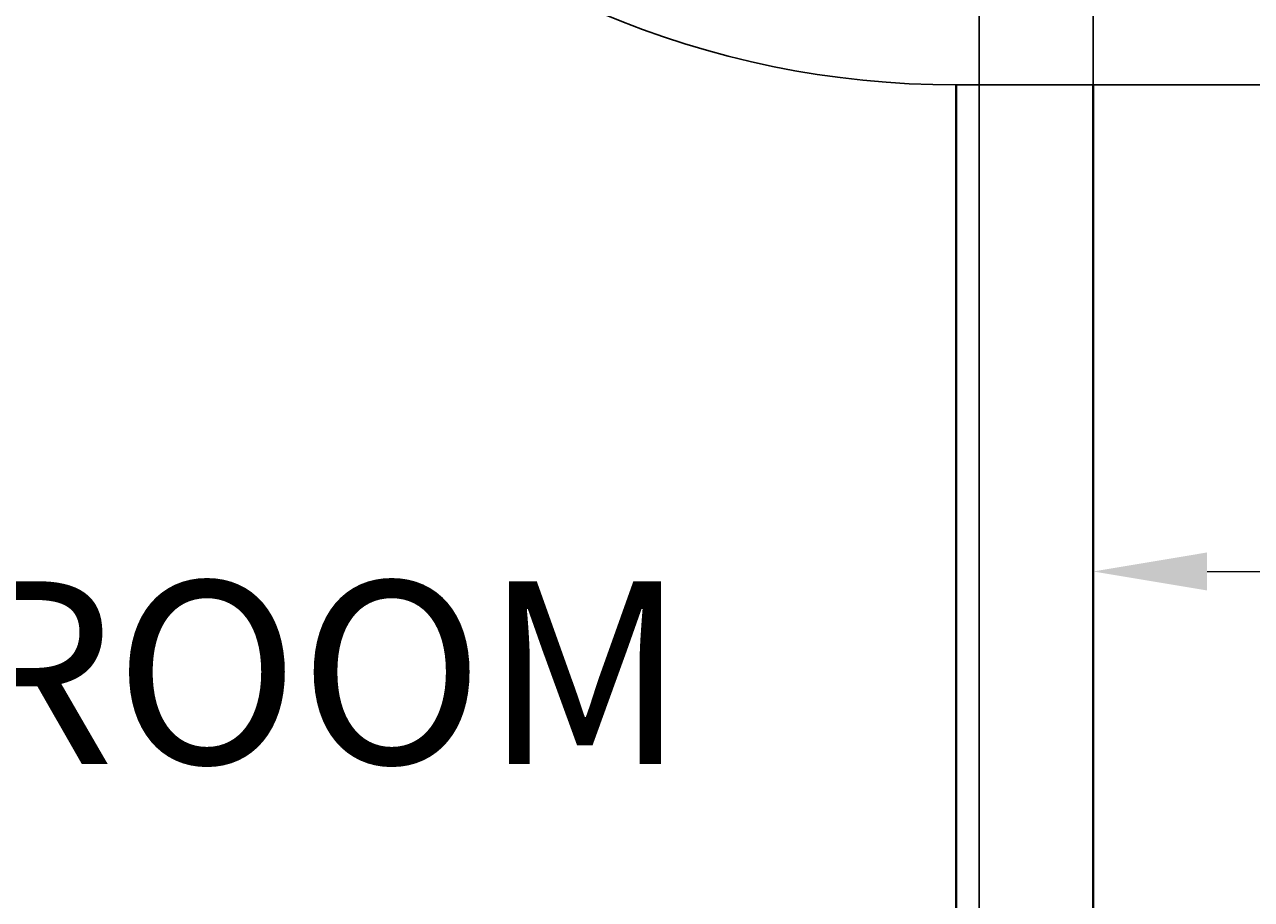
# Model space of a CAD drawing. Units: inches. Extents: x -301 to 715, y -607 to 364.
# Tile 84 of 141: x -92 to -39, y -10 to 28. Entities that reach past the tile are written whole.
import ezdxf

# ---------------------------------------------------------------- set-up
doc = ezdxf.new("R2010")
doc.units = ezdxf.units.IN
doc.header["$MEASUREMENT"] = 0
for name, color, linetype, lineweight in [('A-ANNO-DIMS', 2, 'Continuous', 18), ('A-AREA-IDEN', 220, 'Continuous', 25), ('A-DOOR', 4, 'Continuous', 25), ('A-WALL', 3, 'Continuous', 40)]:
    doc.layers.add(name, color=color, linetype=linetype, lineweight=lineweight)
doc.styles.get("Standard").update_dxf_attribs({"font": 'arial.ttf'})
doc.dimstyles.get("Standard").update_dxf_attribs({"dimtxt": 0.18, "dimasz": 0.18, "dimexe": 0.18, "dimexo": 0.0625, "dimgap": 0.09, "dimtad": 0, "dimtih": 1, "dimtoh": 1, "dimdec": 1, "dimzin": 0, "dimdsep": 46, "dimlunit": 4, "dimtxsty": 'Standard', "dimcen": 0.09, "dimclrd": 3, "dimclre": 4, "dimclrt": 6, "dimadec": 0, "dimazin": 0, "dimtfac": 1, "dimtdec": 1, "dimtofl": 0, "dimtmove": 0, "dimatfit": 3, "dimfxl": 1, "dimtfill": 2, "dimtfillclr": 51, "dimtolj": 1, "dimtzin": 0, "dimarcsym": 0})

# ---------------------------------------------------------------- blocks, each defined once
blk = doc.blocks.new('*U5')
for p, q in [((0, 0), (0, -6)), ((-40, 0), (-40, -6))]:
    blk.add_line(p, q)
blk.add_lwpolyline([(0, 0), (0, 40), (-1.75, 40), (-1.75, 0)], close=True)
blk.add_arc((0, 0), 40, 90, 180)
blk = doc.blocks.new('*D48')
at = {"layer": 'A-ANNO-DIMS', "color": 0, "lineweight": -2, "transparency": 16777216}
for p, q in [((-45.603, -7.657), (-45.603, 4.543)), ((122.71, -8.548), (122.71, 4.543))]:
    blk.add_line(p, q, dxfattribs=at)
at = {"layer": 'A-ANNO-DIMS', "color": 0, "lineweight": 0, "transparency": 16777216}
for p, q in [((-40.603, 4.363), (32.358, 4.363)), ((117.71, 4.363), (44.749, 4.363))]:
    blk.add_line(p, q, dxfattribs=at)
at = {"layer": 'A-ANNO-DIMS', "color": 0, "transparency": 16777216}
for points in [[(-40.603, 5.197), (-40.603, 3.53), (-45.603, 4.363)], [(117.71, 5.197), (117.71, 3.53), (122.71, 4.363)]]:
    blk.add_solid(points, dxfattribs=at)
at = {"layer": 'Defpoints', "color": 0, "transparency": 16777216}
for p in [(-45.603, 4.363), (-45.603, -7.72), (122.71, -8.61)]:
    blk.add_point(p, dxfattribs=at)
at = {"layer": 'A-ANNO-DIMS', "color": 0, "transparency": 16777216, "insert": (38.553, 4.363), "char_height": 3, "attachment_point": 5, "bg_fill": 1, "box_fill_scale": 1.25, "bg_fill_color": 51, "bg_fill_transparency": 0}
blk.add_mtext('\\A1;14\'-0{\\H1x;\\S1/2;}"', dxfattribs=at)
blk = doc.blocks.new('*D149')
at = {"layer": 'A-ANNO-DIMS', "color": 4, "lineweight": -2, "transparency": 16777216}
for p, q in [((-51.541, 65.682), (233.659, 65.682)), ((-51.541, 25.682), (233.659, 25.682))]:
    blk.add_line(p, q, dxfattribs=at)
at = {"layer": 'A-ANNO-DIMS', "color": 3, "lineweight": -2, "transparency": 16777216}
for p, q in [((233.479, 65.502), (233.479, 45.864)), ((233.479, 25.862), (233.479, 45.5))]:
    blk.add_line(p, q, dxfattribs=at)
at = {"layer": 'A-ANNO-DIMS', "color": 3, "transparency": 16777216}
for points in [[(233.449, 65.502), (233.509, 65.502), (233.479, 65.682)], [(233.449, 25.862), (233.509, 25.862), (233.479, 25.682)]]:
    blk.add_solid(points, dxfattribs=at)
at = {"layer": 'Defpoints', "color": 0, "transparency": 16777216}
for p in [(-51.603, 65.682), (-51.603, 25.682), (233.479, 25.682)]:
    blk.add_point(p, dxfattribs=at)
at = {"layer": 'A-ANNO-DIMS', "color": 6, "transparency": 16777216, "insert": (233.479, 45.682), "char_height": 0.18, "attachment_point": 5, "bg_fill": 1, "box_fill_scale": 1.25, "bg_fill_color": 51, "bg_fill_transparency": 0}
blk.add_mtext('\\A1;3\'-4"', dxfattribs=at)
blk = doc.blocks.new('*D151')
at = {"layer": 'A-ANNO-DIMS', "color": 4, "lineweight": -2, "transparency": 16777216}
for p, q in [((-204.603, -223.755), (-204.603, 359.612)), ((-45.603, -214.755), (-45.603, 359.612))]:
    blk.add_line(p, q, dxfattribs=at)
at = {"layer": 'A-ANNO-DIMS', "color": 3, "lineweight": -2, "transparency": 16777216}
for p, q in [((-204.423, 359.432), (-125.494, 359.432)), ((-45.783, 359.432), (-124.713, 359.432))]:
    blk.add_line(p, q, dxfattribs=at)
at = {"layer": 'A-ANNO-DIMS', "color": 3, "transparency": 16777216}
for points in [[(-204.423, 359.462), (-204.423, 359.402), (-204.603, 359.432)], [(-45.783, 359.462), (-45.783, 359.402), (-45.603, 359.432)]]:
    blk.add_solid(points, dxfattribs=at)
at = {"layer": 'Defpoints', "color": 0, "transparency": 16777216}
for p in [(-45.603, 359.432), (-45.603, -214.818), (-204.603, -223.818)]:
    blk.add_point(p, dxfattribs=at)
at = {"layer": 'A-ANNO-DIMS', "color": 6, "transparency": 16777216, "insert": (-125.103, 359.432), "char_height": 0.18, "attachment_point": 5, "bg_fill": 1, "box_fill_scale": 1.25, "bg_fill_color": 51, "bg_fill_transparency": 0}
blk.add_mtext('\\A1;13\'-3"', dxfattribs=at)
blk = doc.blocks.new('*D158')
at = {"layer": 'A-ANNO-DIMS', "color": 4, "lineweight": -2, "transparency": 16777216}
for p, q in [((-122.603, 221.62), (-122.603, -296.865)), ((-50.603, 221.62), (-50.603, -296.865))]:
    blk.add_line(p, q, dxfattribs=at)
at = {"layer": 'A-ANNO-DIMS', "color": 3, "lineweight": -2, "transparency": 16777216}
for p, q in [((-122.423, -296.685), (-86.933, -296.685)), ((-50.783, -296.685), (-86.274, -296.685))]:
    blk.add_line(p, q, dxfattribs=at)
at = {"layer": 'A-ANNO-DIMS', "color": 3, "transparency": 16777216}
for points in [[(-122.423, -296.655), (-122.423, -296.715), (-122.603, -296.685)], [(-50.783, -296.655), (-50.783, -296.715), (-50.603, -296.685)]]:
    blk.add_solid(points, dxfattribs=at)
at = {"layer": 'Defpoints', "color": 0, "transparency": 16777216}
for p in [(-122.603, 221.682), (-50.603, 221.682), (-50.603, -296.685)]:
    blk.add_point(p, dxfattribs=at)
at = {"layer": 'A-ANNO-DIMS', "color": 6, "transparency": 16777216, "insert": (-86.603, -296.685), "char_height": 0.18, "attachment_point": 5, "bg_fill": 1, "box_fill_scale": 1.25, "bg_fill_color": 51, "bg_fill_transparency": 0}
blk.add_mtext('\\A1;6\'-0"', dxfattribs=at)

msp = doc.modelspace()

# ---------------------------------------------------------------- linework, layer by layer
at = {"layer": 'A-WALL'}
for p, q in [((-51.603, -67.318), (-51.603, 25.682)), ((-45.603, -73.318), (-45.603, 25.682))]:
    msp.add_line(p, q, dxfattribs=at)

# ---------------------------------------------------------------- block references
at = {"layer": 'A-DOOR', "rotation": 90}
msp.add_blockref('*U5', (-51.603, 65.682), dxfattribs=at)

# ---------------------------------------------------------------- texts
at = {"layer": 'A-AREA-IDEN', "insert": (-116.542, 3.934), "char_height": 8, "attachment_point": 1}
msp.add_mtext_dynamic_manual_height_columns('BEDROOM', width=73.06001, gutter_width=1, heights=[0], dxfattribs=at)

# ---------------------------------------------------------------- dimensions: what is measured, and where the dimension line sits
at = {"layer": 'A-ANNO-DIMS'}
for base, p1, p2, override, picture, middle in [((-45.603, 359.432), (-204.603, -223.818), (-45.603, -214.818), {"dimdec": 1, "dimlfac": 1, "dimrnd": 0, "dimzin": 1, "dimdsep": 46, "dimlunit": 4, "dimfrac": 2}, '*D151', (-125.103, 359.432)), ((-50.603, -296.685), (-122.603, 221.682), (-50.603, 221.682), {"dimdec": 1, "dimlfac": 1, "dimrnd": 0, "dimzin": 1, "dimdsep": 46, "dimlunit": 4, "dimfrac": 2}, '*D158', (-86.603, -296.685)), ((-45.603, 4.363), (122.71, -8.61), (-45.603, -7.72), {"dimtxt": 3, "dimasz": 5, "dimclrd": 0, "dimclre": 0, "dimclrt": 0, "dimlwd": 0}, '*D48', (38.553, 4.363))]:
    dim = msp.add_linear_dim(base=base, p1=p1, p2=p2, dimstyle='Standard', override=override, dxfattribs=at)
    dim.commit()
    dim.dimension.update_dxf_attribs({"geometry": picture, "text_midpoint": middle})
dim = msp.add_linear_dim(base=(233.479, 25.682), p1=(-51.603, 65.682), p2=(-51.603, 25.682), angle=90, dimstyle='Standard', override={"dimdec": 1, "dimlfac": 1, "dimrnd": 0, "dimzin": 1, "dimdsep": 46, "dimlunit": 4, "dimfrac": 2}, dxfattribs=at)
dim.commit()
dim.dimension.update_dxf_attribs({"geometry": '*D149', "text_midpoint": (233.479, 45.682)})

doc.saveas('drawing.dxf')
